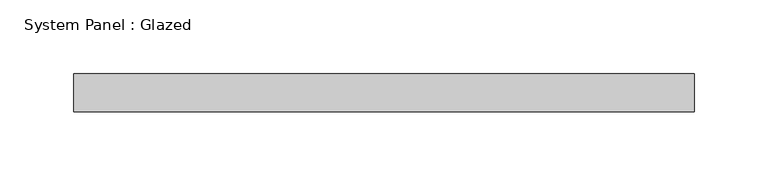
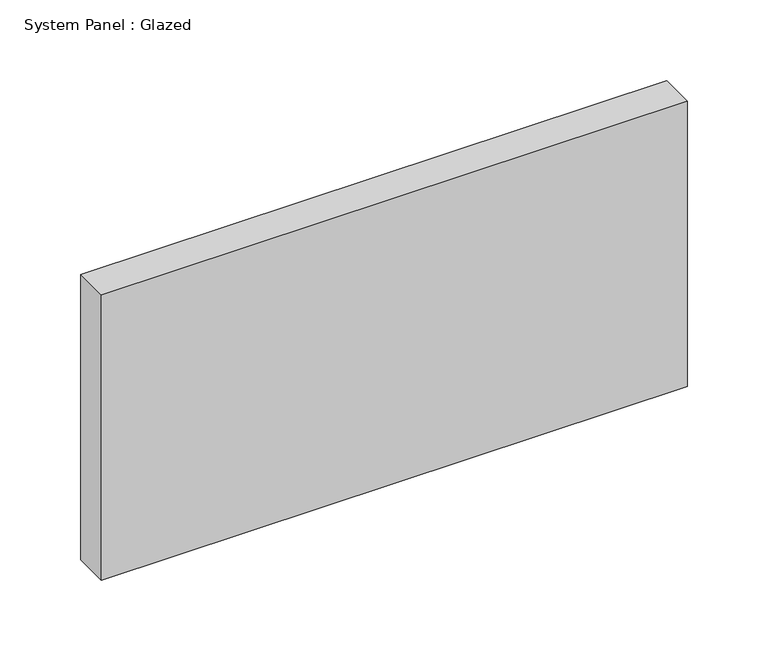
"""IFC4 building model written with IfcOpenShell, lengths in millimetres: plate geometry, System Panel : Glazed."""

from ifc_helpers import new_model, si_unit, origin, origin_with_axes, place, context, project, spatial, polyline, outline, extrude, source, transform, mapped, element, save


def system_panel_glazed_b006000b(model_context):
    return source(origin(), model_context, "Body", "SweptSolid", [
        extrude(outline(polyline([(209.55, 19.05), (-209.55, 19.05), (-209.55, 44.45), (209.55, 44.45), (209.55, 19.05)])), origin_with_axes(), (0.0, 0.0, 1.0), 215.9),
    ])


if __name__ == "__main__":
    model = new_model("IFC4")
    model_context = context("Model", 3, world=origin())
    ifc_project = project(units=[si_unit("LENGTHUNIT", "METRE", prefix="MILLI")], contexts=[model_context])
    site = spatial("IfcSite", under=ifc_project)
    building = spatial("IfcBuilding", under=site)
    placement = place(None, origin())
    system_panel_glazed_shape = system_panel_glazed_b006000b(model_context)
    element("IfcPlate", 1, ObjectType="System Panel : Glazed", at=placement, inside=building, context=model_context, shape_type="MappedRepresentation", body=[
        mapped(system_panel_glazed_shape, transform((0.0, 0.0, 0.0), x_axis=(1.0, 0.0, 0.0), y_axis=(0.0, 1.0, 0.0), z_axis=(0.0, 0.0, 1.0))),
    ])
    save(model, "model.ifc")

# Revit data of these elements
# Type "System Panel : Glazed"
#   Construction Type Id = "GSP4R"
#   Analytic Construction = "1/8 in Pilkington single glazing"
#   Visual Light Transmittance = 0.9
#   Solar Heat Gain Coefficient = 0.86
#   Heat Transfer Coefficient (U) = 1.18115 BTU/(h·ft²·°F)
#   Define Thermal Properties by = 1
# Element 1 (IfcPlate, "System Panel : Glazed")
#   Materials on its faces: "Glass"
# Materials
#   "Glass": class "Glass", colour RGB 0 128 192, transparency 0.75, Description = "Soda Lime Glass", Cost = 0
